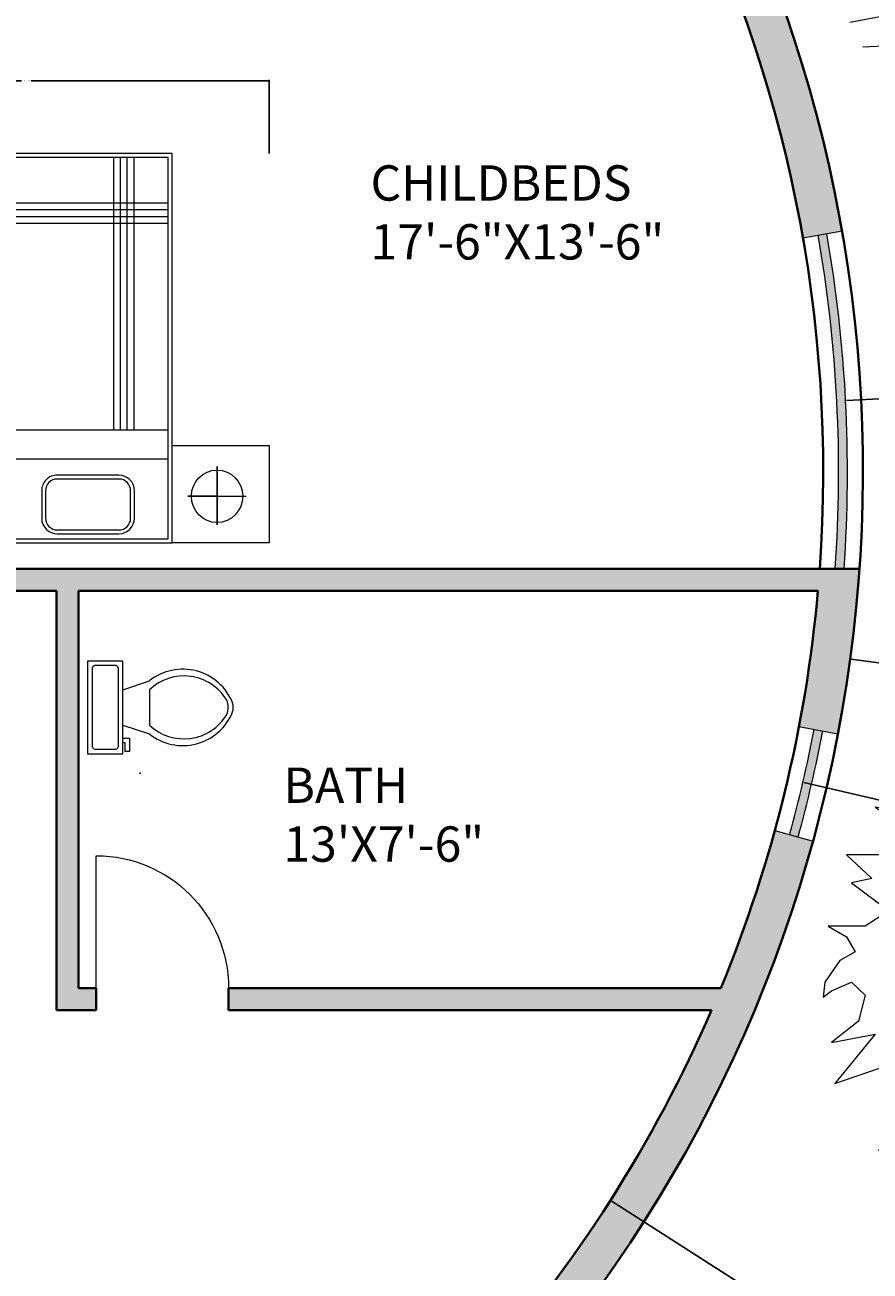
# Model space of a CAD drawing. Units: inches. Extents: x 2330 to 3943, y 1763 to 3461.
# Tile 22 of 40: x 3231 to 3423, y 2547 to 2829. Entities that reach past the tile are written whole.
import ezdxf

# ---------------------------------------------------------------- set-up
doc = ezdxf.new("R2010")
doc.units = ezdxf.units.IN
for name, color, linetype, lineweight in [('A-ANNO-DIMS', 2, 'Continuous', 18), ('A-AREA-IDEN', 7, 'Continuous', 18), ('A-DOOR', 4, 'Continuous', 18), ('A-FLOR-FIXT', 8, 'Continuous', 18), ('A-FURN', 8, 'Continuous', 13), ('A-GLAZ', 4, 'Continuous', 18), ('A-WALL', 7, 'Continuous', 40), ('A-WALL-PATT', 252, 'Continuous', 13), ('L-PLNT', 94, 'Continuous', 13)]:
    doc.layers.add(name, color=color, linetype=linetype, lineweight=lineweight)
doc.styles.get("Standard").update_dxf_attribs({"font": 'arial.ttf'})
doc.dimstyles.get("Standard").update_dxf_attribs({"dimtxt": 0.18, "dimasz": 0.18, "dimexe": 0.18, "dimexo": 0.0625, "dimgap": 0.09, "dimtad": 0, "dimtih": 1, "dimtoh": 1, "dimdec": 4, "dimzin": 0, "dimdsep": 46, "dimtxsty": 'Standard', "dimcen": 0.09, "dimadec": 0, "dimazin": 0, "dimtfac": 1, "dimtdec": 4, "dimtofl": 0, "dimtmove": 0, "dimatfit": 3, "dimfxl": 1, "dimtolj": 1, "dimtzin": 0, "dimarcsym": 0})

# ---------------------------------------------------------------- blocks, each defined once
blk = doc.blocks.new('*U9')
for p, q in [((9.5, -6), (9.5, -2)), ((-8, -8.5), (-8, -8)), ((-7, -8), (-7, -9.5)), ((-4, -8), (-6, -14)), ((4, -8), (6, -14)), ((-10, -8.5), (-8, -8.5)), ((-10, -9.5), (-10, -8.5)), ((-7, -9.5), (-10, -9.5)), ((4, -14), (-4, -14))]:
    blk.add_line(p, q)
blk.add_lwpolyline([(10.5, -8), (10.5, 0), (-10.5, 0), (-10.5, -8)], close=True)
for points in [[(-9.5, -2), (-9.5, -6)], [(8.5, -1), (-8.5, -1)], [(-8.5, -7), (8.5, -7)]]:
    blk.add_lwpolyline(points)
for centre, radius, start, end in [((-8.62, -1.88), 0.884, 81.8699, 188.1301), ((8.62, -1.88), 0.884, 351.8699, 98.1301), ((-8.62, -6.12), 0.884, 171.8699, 278.1301), ((8.62, -6.12), 0.884, 261.8699, 8.1301), ((3.52, -21.58), 12.17, 141.4691, 247.9714), ((4.2, -21.82), 11.33, 136.3677, 238.9468), ((-3.52, -21.58), 12.17, 292.0284, 38.5307), ((-4.2, -21.82), 11.33, 301.053, 43.6321), ((0, -27.88), 4, 245.7318, 294.2682), ((0, -29), 4, 254.8605, 285.1395)]:
    blk.add_arc(centre, radius, start, end)
blk = doc.blocks.new('A$C057D194F')
for p, q in [((0, 1.5, -0.1688), (0, 2, -0.1688)), ((0, 2, -0.1688), (0.5, 2, -0.1688)), ((0.5, 2, -0.1688), (0.5, 0, -0.1688)), ((2, 2, -0.1688), (0.5, 2, -0.1688)), ((2, 0, -0.1688), (2, 2, -0.1688)), ((2.5, 2, -0.1688), (2, 2, -0.1688)), ((2.5, 1.5, -0.1688), (2.5, 2, -0.1688)), ((1.98, 1.98, -0.1688), (0.52, 1.98, -0.1688)), ((0.52, 1.98, -0.1688), (0.52, 0.02, -0.1688)), ((1.0907, 1.9539, -0.1688), (0.7735, 1.9539, -0.1688)), ((1.0907, 1.9339, -0.1688), (0.7735, 1.9339, -0.1688)), ((1.8224, 1.9539, -0.1688), (1.5052, 1.9539, -0.1688)), ((1.8224, 1.9339, -0.1688), (1.5052, 1.9339, -0.1688)), ((1.98, 0.02, -0.1688), (1.98, 1.98, -0.1688)), ((0.2687, 1.9081, -0.1688), (0.2687, 1.761, -0.1688)), ((0.2687, 1.6081, -0.1688), (0.2687, 1.9081, -0.1688)), ((0.6935, 1.8739, -0.1688), (0.6935, 1.7322, -0.1688)), ((0.7135, 1.8739, -0.1688), (0.7135, 1.7322, -0.1688)), ((1.1507, 1.7322, -0.1688), (1.1507, 1.8739, -0.1688)), ((1.1707, 1.7322, -0.1688), (1.1707, 1.8739, -0.1688)), ((1.4252, 1.8739, -0.1688), (1.4252, 1.7322, -0.1688)), ((1.4452, 1.8739, -0.1688), (1.4452, 1.7322, -0.1688)), ((1.8824, 1.7322, -0.1688), (1.8824, 1.8739, -0.1688)), ((1.9024, 1.7322, -0.1688), (1.9024, 1.8739, -0.1688)), ((2.2313, 1.9081, -0.1688), (2.2313, 1.761, -0.1688)), ((2.2313, 1.6081, -0.1688), (2.2313, 1.9081, -0.1688)), ((0.4194, 1.761, -0.1688), (0.1194, 1.761, -0.1688)), ((0.2687, 1.761, -0.1688), (0.4194, 1.761, -0.1688)), ((0.2687, 1.761, -0.1688), (0.2687, 1.6081, -0.1688)), ((2.0806, 1.761, -0.1688), (2.3806, 1.761, -0.1688)), ((2.2313, 1.761, -0.1688), (2.0806, 1.761, -0.1688)), ((2.2313, 1.761, -0.1688), (2.2313, 1.6081, -0.1688)), ((0.7735, 1.6722, -0.1688), (1.0907, 1.6722, -0.1688)), ((1.5052, 1.6722, -0.1688), (1.8224, 1.6722, -0.1688)), ((0.7735, 1.6522, -0.1688), (1.0907, 1.6522, -0.1688)), ((1.5052, 1.6522, -0.1688), (1.8224, 1.6522, -0.1688)), ((1.98, 1.5693, -0.1688), (0.52, 1.5693, -0.1688)), ((0.5, 1.5, -0.1688), (0, 1.5, -0.1688)), ((2, 1.5, -0.1688), (2.5, 1.5, -0.1688)), ((1.98, 1.4193, -0.1688), (0.52, 1.4193, -0.1688)), ((0.6969, 0.02, -0.1688), (0.6969, 1.4193, -0.1688)), ((0.7319, 0.02, -0.1688), (0.7319, 1.4193, -0.1688)), ((0.7669, 0.02, -0.1688), (0.7669, 1.4193, -0.1688)), ((0.8019, 0.02, -0.1688), (0.8019, 1.4193, -0.1688)), ((0.52, 0.3595, -0.1688), (1.9292, 0.3595, -0.1688)), ((0.52, 0.3245, -0.1688), (1.905, 0.3245, -0.1688)), ((0.52, 0.2895, -0.1688), (1.8742, 0.2895, -0.1688)), ((0.52, 0.2545, -0.1688), (1.8344, 0.2545, -0.1688)), ((1.6548, 0.1789, -0.1688), (1.7198, 0.0251, -0.1688)), ((0.52, 0.02, -0.1688), (1.98, 0.02, -0.1688)), ((0.5, 0, -0.1688), (2, 0, -0.1688))]:
    blk.add_line(p, q)
for centre, radius, start, end in [((0.7735, 1.8739, -0.1688), 0.08, 90, 180), ((0.7735, 1.8739, -0.1688), 0.06, 90, 180), ((1.0907, 1.8739, -0.1688), 0.08, 0, 90), ((1.0907, 1.8739, -0.1688), 0.06, 0, 90), ((1.5052, 1.8739, -0.1688), 0.08, 90, 180), ((1.5052, 1.8739, -0.1688), 0.06, 90, 180), ((1.8224, 1.8739, -0.1688), 0.08, 0, 90), ((1.8224, 1.8739, -0.1688), 0.06, 0, 90), ((0.7735, 1.7322, -0.1688), 0.08, 180, 270), ((0.7735, 1.7322, -0.1688), 0.06, 180, 270), ((1.0907, 1.7322, -0.1688), 0.08, 270, 0), ((1.0907, 1.7322, -0.1688), 0.06, 270, 0), ((1.5052, 1.7322, -0.1688), 0.08, 180, 270), ((1.5052, 1.7322, -0.1688), 0.06, 180, 270), ((1.8224, 1.7322, -0.1688), 0.08, 270, 0), ((1.8224, 1.7322, -0.1688), 0.06, 270, 0), ((1.5992, 0.5623, -0.1688), 0.3874, 278.2518, 356.6808), ((1.363, 0.5286, -0.1688), 0.6171, 305.32946, 1.04595)]:
    blk.add_arc(centre, radius, start, end)
blk.add_ellipse((0.2687, 1.761, -0.1688), major_axis=(0, -0.1351), ratio=0.975448)
at = {"extrusion": (0, 0, -1)}
blk.add_ellipse((2.2313, 1.761, -0.1688), major_axis=(0, 0.1351), ratio=0.975448, dxfattribs=at)
for p in [(0.2687, 1.761, -0.1688), (2.2313, 1.761, -0.1688)]:
    blk.add_point(p)
blk = doc.blocks.new('*U12')
for p, q in [((0, 0), (-10.5, 57)), ((-10.186, 53.64), (-13.084, 55.962)), ((-9.099, 51.782), (-6.563, 55.962)), ((-8.737, 47.138), (-17.069, 52.711)), ((-7.65, 43.423), (-2.578, 49.46)), ((-5.839, 35.992), (4.667, 48.067)), ((-7.288, 39.707), (-21.778, 46.673)), ((-5.114, 27.632), (10.463, 46.673)), ((-5.114, 28.097), (-24.676, 40.636)), ((-2.941, 16.486), (8.652, 37.85)), ((-3.665, 19.273), (-27.574, 35.527)), ((27, 9), (48, 36)), ((27.127, 9.056), (31.112, 35.992)), ((38.719, 34.134), (41.979, 28.561)), ((44.153, 36.456), (45.239, 32.741)), ((16.259, 5.805), (23.142, 31.348)), ((22.055, 7.198), (27.489, 32.277)), ((35.096, 32.741), (37.27, 22.524)), ((-48.585, 21.131), (-49.309, 29.026)), ((-43.513, 28.561), (-42.427, 15.558)), ((31.836, 30.883), (32.561, 16.486)), ((43.791, 29.954), (51.036, 30.883)), ((-31.5, 4.5), (-52.5, 25.5)), ((-38.442, 26.239), (-34.819, 7.663)), ((-35.544, 28.097), (-24.314, 3.947)), ((-1.129, 6.734), (9.014, 26.704)), ((10.101, 3.483), (17.708, 26.239)), ((40.53, 25.775), (48.862, 24.846)), ((-14.533, 2.09), (-30.834, 25.31)), ((-24.314, 23.917), (-2.941, 13.7)), ((3.942, 1.625), (11.187, 24.381)), ((-47.498, 19.737), (-55.83, 18.344)), ((36.183, 19.737), (48.137, 17.88)), ((33.285, 16.486), (48.862, 10.913)), ((-40.615, 13.7), (-55.105, 10.913)), ((-20.691, 13.7), (-1.129, 4.876)), ((29.662, 12.307), (48.137, 6.269)), ((0, 0), (27, 9)), ((-33.37, 6.269), (-52.207, 5.34)), ((18.07, 5.805), (35.096, -3.483)), ((24.229, 7.663), (46.688, 1.625)), ((-28.299, 3.483), (-47.86, -5.805)), ((-21.416, 3.018), (-38.079, -8.128)), ((0, 0), (-31.5, 4.5)), ((11.187, 3.483), (30.749, -5.805)), ((-15.982, 2.09), (-30.11, -9.521)), ((0, 0), (-22.5, -19.5)), ((-6.563, 1.161), (-21.416, -8.128)), ((0, 0), (18, -22.5)), ((6.478, 1.625), (26.04, -8.592)), ((1.769, -2.555), (24.229, -9.521)), ((-4.752, -3.483), (-3.665, -14.629)), ((2.493, -3.019), (-1.491, -20.202)), ((-6.563, -5.805), (-19.967, -9.985)), ((5.029, -6.27), (2.131, -25.775)), ((-9.461, -8.592), (-6.201, -23.453)), ((7.565, -9.056), (32.198, -14.629)), ((-15.257, -12.772), (-30.11, -12.772)), ((-13.446, -11.378), (-8.737, -32.741)), ((9.014, -11.378), (3.58, -35.992)), ((-17.431, -15.094), (-42.789, -18.809)), ((-17.069, -15.094), (-12.721, -40.172)), ((12.274, -15.094), (36.907, -18.809)), ((-22.5, -19.5), (-37.5, -45)), ((-20.691, -18.345), (-17.793, -44.352)), ((14.085, -16.951), (6.478, -40.172)), ((16.259, -19.738), (36.183, -22.989)), ((-24.314, -21.596), (-42.427, -22.06)), ((18.07, -22.524), (8.289, -45.745)), ((18, -22.5), (27, -52.5)), ((18.433, -22.524), (40.53, -29.026)), ((-25.038, -23.918), (-22.865, -45.281)), ((19.157, -25.311), (38.719, -33.206)), ((-26.849, -26.24), (-40.253, -25.775)), ((-28.299, -29.026), (-42.789, -31.348)), ((-29.023, -30.884), (-27.936, -43.887)), ((20.244, -30.419), (15.897, -44.816)), ((21.331, -32.741), (39.081, -40.636)), ((-30.834, -34.135), (-42.427, -35.528)), ((-32.646, -36.921), (-31.921, -44.352)), ((22.78, -37.85), (19.519, -48.532)), ((22.78, -38.314), (34.372, -44.816)), ((-34.457, -39.708), (-40.978, -42.494)), ((24.591, -43.423), (30.749, -47.603)), ((24.591, -45.745), (23.142, -50.854)), ((26.764, -49.925), (28.213, -50.854))]:
    blk.add_line(p, q)
blk = doc.blocks.new('*U15')
for points in [[(0, 60.64), (-3.051, 56.238), (-4.196, 52.815), (-5.34, 47.925), (-6.103, 45.969), (-11.062, 50.859), (-18.691, 52.326), (-20.98, 47.436), (-20.217, 43.524), (-20.598, 39.611), (-25.939, 43.035), (-27.846, 49.392), (-33.186, 52.326), (-30.516, 47.436), (-31.279, 43.035), (-30.135, 38.144), (-33.568, 35.21), (-40.815, 36.677), (-49.208, 38.144), (-46.919, 36.677), (-42.341, 31.787), (-42.341, 28.364), (-46.537, 27.386), (-55.692, 27.386), (-49.97, 22.006), (-54.548, 21.028), (-46.156, 14.671), (-51.496, 11.248), (-59.888, 11.248), (-55.692, 8.803), (-53.785, 5.38), (-57.218, 3.423), (-60.651, -1.467), (-61.033, -4.89), (-59.125, -3.423), (-54.548, -1.467), (-51.496, -4.401), (-53.022, -10.269), (-59.125, -15.16), (-49.208, -13.204), (-58.362, -24.451), (-48.445, -21.028), (-43.486, -22.495), (-43.104, -25.918), (-47.3, -31.298), (-43.104, -30.32), (-48.445, -39.611), (-38.527, -31.787), (-40.815, -36.188), (-32.423, -37.166), (-33.568, -43.523), (-35.475, -49.392), (-28.609, -44.99), (-23.65, -46.457), (-22.124, -51.837), (-21.743, -57.705), (-19.073, -52.326), (-15.639, -51.837), (-12.588, -58.683), (-11.062, -54.771), (-6.866, -49.392), (-6.866, -53.304), (-4.959, -48.414), (-1.907, -61.617), (-1.144, -51.348), (4.578, -59.172), (5.341, -54.282), (9.918, -56.727), (12.207, -60.639), (12.97, -47.925), (14.877, -44.501), (17.547, -47.436), (19.455, -52.815), (22.888, -60.639), (21.743, -49.392), (23.65, -46.457), (29.754, -47.925), (35.094, -52.326), (37.001, -53.793), (33.187, -46.457), (32.042, -41.567), (35.094, -39.122), (43.868, -40.589), (47.682, -42.056), (43.105, -36.188), (43.105, -33.743), (46.538, -31.298), (50.352, -32.765), (46.919, -26.407), (55.693, -22.495), (60.652, -22.984), (66.374, -22.006), (59.889, -20.05), (54.167, -18.094), (51.878, -15.649), (49.589, -12.225), (51.497, -10.269), (57.981, -9.78), (63.322, -7.335), (64.466, -2.934)], [(64.848, -2.934), (59.507, -5.379), (56.456, -4.401), (51.878, -2.445), (52.26, 0.978), (55.311, 3.912), (59.889, 5.869), (62.94, 11.248), (58.363, 10.27), (54.548, 10.27), (51.115, 11.248), (53.785, 15.649), (57.981, 18.094), (60.652, 19.561), (56.074, 19.561), (51.115, 17.605), (46.538, 19.072), (46.156, 22.496), (49.589, 27.386), (52.26, 34.721), (49.589, 33.743), (44.249, 30.32), (41.197, 32.276), (41.579, 37.655), (43.868, 42.546), (43.105, 46.947), (40.053, 44.013), (36.238, 40.589), (33.568, 42.057), (33.95, 45.969), (35.476, 52.815), (31.28, 49.392), (26.702, 46.947), (28.228, 50.859), (28.609, 61.129), (24.795, 54.282), (18.692, 50.859), (17.929, 57.706), (12.97, 50.859), (7.248, 57.706), (5.341, 53.304), (0, 60.64)]]:
    blk.add_lwpolyline(points)
blk.add_lwpolyline([(0.382, 1.956), (0, 0), (1.907, 0.489), (2.289, 1.467)], close=True)
blk = doc.blocks.new('DOOR-SINGLE-30IN')
blk.add_line((0, 0), (0, 30))
blk.add_arc((0, 0), 30, 90, 180)
blk = doc.blocks.new('*D57')
at = {"layer": 'A-ANNO-DIMS', "color": 0, "lineweight": -2, "transparency": 16777216}
for p, q in [((3176.71, 2799.74), (3176.71, 2816.38)), ((3176.89, 2816.2), (3230.73, 2816.2)), ((3286.72, 2816.2), (3232.88, 2816.2)), ((3286.9, 2799.74), (3286.9, 2816.38))]:
    blk.add_line(p, q, dxfattribs=at)
at = {"layer": 'A-ANNO-DIMS', "color": 0, "transparency": 16777216}
for points in [[(3176.89, 2816.23), (3176.89, 2816.17), (3176.71, 2816.2)], [(3286.72, 2816.23), (3286.72, 2816.17), (3286.9, 2816.2)]]:
    blk.add_solid(points, dxfattribs=at)
at = {"layer": 'Defpoints', "color": 0, "transparency": 16777216}
for p in [(3176.71, 2816.2), (3176.71, 2799.68), (3286.9, 2799.68)]:
    blk.add_point(p, dxfattribs=at)
at = {"layer": 'A-ANNO-DIMS', "color": 0, "transparency": 16777216, "insert": (3231.8, 2816.2), "char_height": 0.18, "attachment_point": 5}
blk.add_mtext('\\A1;SINGLE BED 110', dxfattribs=at)
blk = doc.blocks.new('*D95')
at = {"layer": 'A-ANNO-DIMS', "color": 0, "lineweight": -2, "transparency": 16777216}
for p, q in [((3105.6, 2727.69), (3105.78, 2727.69)), ((3105.69, 2727.6), (3105.69, 2727.78)), ((3606.31, 2659.69), (3418.76, 2685.16))]:
    blk.add_line(p, q, dxfattribs=at)
at = {"layer": 'A-ANNO-DIMS', "color": 0, "transparency": 16777216}
blk.add_solid([(3418.76, 2685.19), (3418.75, 2685.14), (3418.58, 2685.19)], dxfattribs=at)
at = {"layer": 'Defpoints', "color": 0, "transparency": 16777216}
for p in [(3105.69, 2727.69), (3418.58, 2685.19)]:
    blk.add_point(p, dxfattribs=at)
at = {"layer": 'A-ANNO-DIMS', "color": 0, "transparency": 16777216, "insert": (3606.86, 2659.69), "char_height": 0.18, "attachment_point": 5}
blk.add_mtext('\\A1;R315.76', dxfattribs=at)
blk = doc.blocks.new('*D96')
at = {"layer": 'A-ANNO-DIMS', "color": 0, "lineweight": -2, "transparency": 16777216}
for p, q in [((3604.65, 2753.34), (3417.72, 2743.73)), ((3105.6, 2727.69), (3105.78, 2727.69)), ((3105.69, 2727.6), (3105.69, 2727.78))]:
    blk.add_line(p, q, dxfattribs=at)
at = {"layer": 'A-ANNO-DIMS', "color": 0, "transparency": 16777216}
blk.add_solid([(3417.72, 2743.76), (3417.72, 2743.7), (3417.54, 2743.72)], dxfattribs=at)
at = {"layer": 'Defpoints', "color": 0, "transparency": 16777216}
for p in [(3417.54, 2743.72), (3105.69, 2727.69)]:
    blk.add_point(p, dxfattribs=at)
at = {"layer": 'A-ANNO-DIMS', "color": 0, "transparency": 16777216, "insert": (3605.39, 2753.34), "char_height": 0.18, "attachment_point": 5}
blk.add_mtext('\\A1;2X R312.26', dxfattribs=at)
blk = doc.blocks.new('*D97')
at = {"layer": 'A-ANNO-DIMS', "color": 0, "lineweight": -2, "transparency": 16777216}
for p, q in [((3105.6, 2727.69), (3105.78, 2727.69)), ((3105.69, 2727.6), (3105.69, 2727.78)), ((3589.17, 2615.07), (3408.04, 2657.26))]:
    blk.add_line(p, q, dxfattribs=at)
at = {"layer": 'A-ANNO-DIMS', "color": 0, "transparency": 16777216}
blk.add_solid([(3408.05, 2657.29), (3408.03, 2657.23), (3407.86, 2657.3)], dxfattribs=at)
at = {"layer": 'Defpoints', "color": 0, "transparency": 16777216}
for p in [(3105.69, 2727.69), (3407.86, 2657.3)]:
    blk.add_point(p, dxfattribs=at)
at = {"layer": 'A-ANNO-DIMS', "color": 0, "transparency": 16777216, "insert": (3589.91, 2615.07), "char_height": 0.18, "attachment_point": 5}
blk.add_mtext('\\A1;2X R310.26', dxfattribs=at)
blk = doc.blocks.new('*D98')
at = {"layer": 'A-ANNO-DIMS', "color": 0, "lineweight": -2, "transparency": 16777216}
for p, q in [((3105.6, 2727.69), (3105.78, 2727.69)), ((3105.69, 2727.6), (3105.69, 2727.78)), ((3519.33, 2463.49), (3364.37, 2562.47)), ((3519.51, 2463.49), (3519.33, 2463.49))]:
    blk.add_line(p, q, dxfattribs=at)
at = {"layer": 'A-ANNO-DIMS', "color": 0, "transparency": 16777216}
blk.add_solid([(3364.39, 2562.49), (3364.35, 2562.44), (3364.22, 2562.56)], dxfattribs=at)
at = {"layer": 'Defpoints', "color": 0, "transparency": 16777216}
for p in [(3105.69, 2727.69), (3364.22, 2562.56)]:
    blk.add_point(p, dxfattribs=at)
at = {"layer": 'A-ANNO-DIMS', "color": 0, "transparency": 16777216, "insert": (3520.26, 2463.49), "char_height": 0.18, "attachment_point": 5}
blk.add_mtext('\\A1;3X R306.76', dxfattribs=at)
blk = doc.blocks.new('*D103')
at = {"layer": 'A-ANNO-DIMS', "color": 0, "lineweight": -2, "transparency": 16777216}
for p, q in [((3257.55, 2659.32), (3257.73, 2659.32)), ((3257.64, 2659.23), (3257.64, 2659.41)), ((3257.66, 1763.59), (3257.65, 2099.31)), ((3257.84, 1763.59), (3257.66, 1763.59))]:
    blk.add_line(p, q, dxfattribs=at)
at = {"layer": 'A-ANNO-DIMS', "color": 0, "transparency": 16777216}
blk.add_solid([(3257.68, 2099.31), (3257.62, 2099.31), (3257.65, 2099.49)], dxfattribs=at)
at = {"layer": 'Defpoints', "color": 0, "transparency": 16777216}
for p in [(3257.64, 2659.32), (3257.65, 2099.49)]:
    blk.add_point(p, dxfattribs=at)
at = {"layer": 'A-ANNO-DIMS', "color": 0, "transparency": 16777216, "insert": (3258.58, 1763.59), "char_height": 0.18, "attachment_point": 5}
blk.add_mtext('\\A1;40X R559.8', dxfattribs=at)
blk = doc.blocks.new('*D104')
at = {"layer": 'A-ANNO-DIMS', "color": 0, "lineweight": -2, "transparency": 16777216}
for p, q in [((3257.55, 2659.32), (3257.73, 2659.32)), ((3257.64, 2659.23), (3257.64, 2659.41)), ((3257.66, 1917.19), (3257.65, 2195.31)), ((3257.84, 1917.19), (3257.66, 1917.19))]:
    blk.add_line(p, q, dxfattribs=at)
at = {"layer": 'A-ANNO-DIMS', "color": 0, "transparency": 16777216}
blk.add_solid([(3257.68, 2195.31), (3257.62, 2195.31), (3257.65, 2195.49)], dxfattribs=at)
at = {"layer": 'Defpoints', "color": 0, "transparency": 16777216}
for p in [(3257.64, 2659.32), (3257.65, 2195.49)]:
    blk.add_point(p, dxfattribs=at)
at = {"layer": 'A-ANNO-DIMS', "color": 0, "transparency": 16777216, "insert": (3258.58, 1917.19), "char_height": 0.18, "attachment_point": 5}
blk.add_mtext('\\A1;33X R463.8', dxfattribs=at)

msp = doc.modelspace()

# ---------------------------------------------------------------- hatches: boundary and pattern name
at = {"layer": 'A-GLAZ'}
h = msp.add_hatch(color=256, dxfattribs=at)
h.dxf.hatch_style = 1
h.paths.add_polyline_path([(3413.2714, 2781.5552), (3411.3014, 2781.2102, -0.06119073), (3415.1695, 2705.6524), (3417.1745, 2705.6524, 0.0610763)])
h = msp.add_hatch(color=256, dxfattribs=at)
h.dxf.hatch_style = 1
h.paths.add_polyline_path([(3412.3715, 2668.9116), (3410.4073, 2669.288, -0.01975096), (3404.8487, 2645.4247), (3406.7771, 2644.8945, 0.01975096)])
at = {"layer": 'A-WALL-PATT'}
h = msp.add_hatch(color=256, dxfattribs=at)
h.dxf.hatch_style = 1
h.paths.add_polyline_path([(3387.1394, 2870.8379, 0.10459296), (3403.8352, 2898.1524), (3395.3511, 2901.1556, -0.12790871), (3376.0739, 2872.6524), (3241.6605, 2872.6524), (3241.6605, 2876.6524), (3236.6605, 2876.6524), (3236.6605, 2872.6524), (3232.6605, 2872.6524), (3232.6605, 2867.6524), (3378.6605, 2867.6524, -0.07524693), (3407.8539, 2780.6064), (3416.7189, 2782.159, 0.07442358)])
h = msp.add_hatch(color=256, dxfattribs=at)
h.dxf.hatch_style = 1
h.paths.add_polyline_path([(3420.6832, 2705.6524), (3159.6605, 2705.6524), (3159.6605, 2827.6524), (3154.6605, 2827.6524), (3154.6605, 2705.6524), (3017.6605, 2705.6524), (3017.6605, 2700.6524), (3238.6605, 2700.6524), (3238.6605, 2605.6524), (3247.6605, 2605.6524), (3247.6605, 2610.6524), (3243.6605, 2610.6524), (3243.6605, 2700.6524), (3411.2593, 2700.6524, -0.02528333), (3406.9698, 2669.9468), (3415.809, 2668.2528, 0.02988796)])
h = msp.add_hatch(color=256, dxfattribs=at)
h.dxf.hatch_style = 1
h.paths.add_polyline_path([(3410.1519, 2643.9665), (3401.474, 2646.3527, -0.03078214), (3389.25, 2610.6524), (3277.6605, 2610.6524), (3277.6605, 2605.6524), (3387.1343, 2605.6524, -0.07980087), (3334.7596, 2523.6524), (3323.7816, 2523.6524), (3323.7816, 2514.6524), (3338.7607, 2514.6524, 0.11859459)])

# ---------------------------------------------------------------- linework, layer by layer
at = {"layer": 'A-GLAZ'}
for p, q in [((3407.8539, 2780.6064), (3416.7189, 2782.159)), ((3406.9698, 2669.9468), (3415.809, 2668.2528)), ((3401.474, 2646.3527), (3410.1519, 2643.9665))]:
    msp.add_line(p, q, dxfattribs=at)
for radius, start, end in [(310.2595, 355.927452, 9.933869), (312.2595, 355.95358, 9.933869), (310.2595, 344.624731, 349.150728), (312.2595, 344.624731, 349.150728)]:
    msp.add_arc((3105.6935, 2727.6869), radius, start, end, dxfattribs=at)
at = {"layer": 'A-WALL'}
for p, q in [((3159.6605, 2705.6524), (3420.6832, 2705.6524)), ((3017.6605, 2700.6524), (3238.6605, 2700.6524)), ((3238.6605, 2700.6524), (3238.6605, 2605.6524)), ((3243.6605, 2700.6524), (3243.6605, 2610.6524)), ((3243.6605, 2700.6524), (3411.2593, 2700.6524)), ((3243.6605, 2610.6524), (3247.6605, 2610.6524)), ((3247.6605, 2610.6524), (3247.6605, 2605.6524)), ((3277.6605, 2610.6524), (3277.6605, 2605.6524)), ((3277.6605, 2610.6524), (3389.25, 2610.6524)), ((3238.6605, 2605.6524), (3247.6605, 2605.6524)), ((3277.6605, 2605.6524), (3387.1343, 2605.6524))]:
    msp.add_line(p, q, dxfattribs=at)
for radius, start, end in [(315.7595, 317.571214, 26.95911), (306.7595, 355.880906, 27.146756), (306.7595, 337.572212, 354.944006), (306.7595, 318.307811, 336.558149)]:
    msp.add_arc((3105.6935, 2727.6869), radius, start, end, dxfattribs=at)

# ---------------------------------------------------------------- block references
at = {"layer": 'A-DOOR', "extrusion": (0, 0, -1), "zscale": -1}
msp.add_blockref('DOOR-SINGLE-30IN', (-3247.6605, 2610.6524), dxfattribs=at)
at = {"layer": 'A-FLOR-FIXT', "rotation": 90}
msp.add_blockref('*U9', (3245.7203, 2674.246), dxfattribs=at)
at = {"layer": 'A-FURN', "xscale": 44.07393684478161, "yscale": 44.07393684478161, "zscale": 44.07393684478161, "rotation": 180}
msp.add_blockref('A$C057D194F', (3286.8969, 2799.6765, 7.4375), dxfattribs=at)
at = {"layer": 'L-PLNT'}
for name, p in [('*U12', (3473.6244, 2818.4657)), ('*U15', (3473.4568, 2613.4629))]:
    msp.add_blockref(name, p, dxfattribs=at)

# ---------------------------------------------------------------- texts
at = {"layer": 'A-AREA-IDEN', "char_height": 8, "attachment_point": 1}
for s, width, insert in [('CHILDBEDS\\P17\'-6"X13\'-6"', 114.537883, (3309.8423, 2797.0385)), ('BATH\\P13\'X7\'-6"', 69.30651, (3290.0874, 2660.6211))]:
    msp.add_mtext_dynamic_manual_height_columns(s, width=width, gutter_width=12.5, heights=[0], dxfattribs=dict(at, insert=insert))

# ---------------------------------------------------------------- dimensions: what is measured, and where the dimension line sits
at = {"layer": 'A-ANNO-DIMS'}
dim = msp.add_linear_dim(base=(3176.7121, 2816.2042), p1=(3286.8969, 2799.6765), p2=(3176.7121, 2799.6765), angle=180, text='SINGLE BED <>', dimstyle='Standard', override={"dimdec": 0, "dimlfac": 1, "dimrnd": 0, "dimzin": 0, "dimdsep": 46, "dimlunit": 2}, dxfattribs=at)
dim.commit()
dim.dimension.update_dxf_attribs({"geometry": '*D57', "text_midpoint": (3231.8045, 2816.2042)})
for center, mpoint, text, override, picture, middle in [((3105.6935, 2727.6869), (3417.5409, 2743.723), '2X <>', {"dimdec": 2, "dimlfac": 1, "dimrnd": 0, "dimzin": 0, "dimdsep": 46, "dimlunit": 2}, '*D96', (3604.6494, 2753.3446)), ((3105.6935, 2727.6869), (3407.8638, 2657.302), '2X <>', {"dimdec": 2, "dimlfac": 1, "dimrnd": 0, "dimzin": 0, "dimdsep": 46, "dimlunit": 2}, '*D97', (3589.166, 2615.0711)), ((3105.6935, 2727.6869), (3364.219, 2562.563), '3X <>', {"dimdec": 2, "dimlfac": 1, "dimrnd": 0, "dimzin": 0, "dimdsep": 46, "dimlunit": 2}, '*D98', (3520.2574, 2463.4886)), ((3257.6403, 2659.3212), (3257.65, 2099.4902), '40X <>', {"dimdec": 1, "dimlfac": 1, "dimrnd": 0, "dimzin": 0, "dimdsep": 46, "dimlunit": 2}, '*D103', (3258.5828, 1763.5916)), ((3257.6403, 2659.3212), (3257.65, 2195.4902), '33X <>', {"dimdec": 1, "dimlfac": 1, "dimrnd": 0, "dimzin": 0, "dimdsep": 46, "dimlunit": 2}, '*D104', (3258.5791, 1917.1916))]:
    dim = msp.add_radius_dim(center=center, mpoint=mpoint, text=text, dimstyle='Standard', override=override, dxfattribs=at)
    dim.commit()
    dim.dimension.update_dxf_attribs({"geometry": picture, "text_midpoint": middle, "dimtype": 164})
dim = msp.add_radius_dim(center=(3105.6935, 2727.6869), mpoint=(3418.58, 2685.189), dimstyle='Standard', override={"dimdec": 2, "dimlfac": 1, "dimrnd": 0, "dimzin": 0, "dimdsep": 46, "dimlunit": 2}, dxfattribs=at)
dim.commit()
dim.dimension.update_dxf_attribs({"geometry": '*D95', "text_midpoint": (3606.3119, 2659.6902), "dimtype": 164})

doc.saveas('drawing.dxf')
